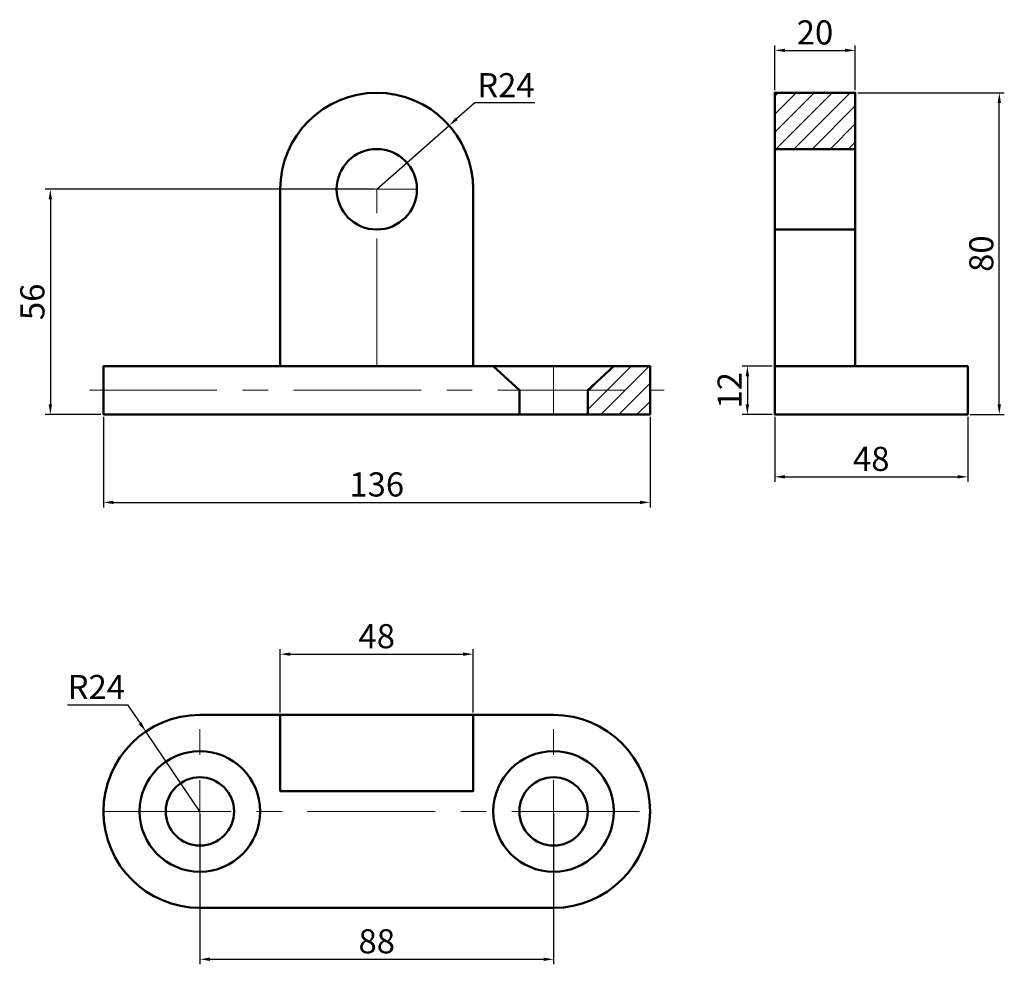
# Model space of a CAD drawing. Units: millimetres. Extents: x 11 to 256, y 19 to 254.
import ezdxf

# ---------------------------------------------------------------- set-up
doc = ezdxf.new("R2010")
doc.units = ezdxf.units.MM
doc.linetypes.add('CENTER', pattern=[50.8, 31.75, -6.35, 6.35, -6.35])
for name, color, linetype, lineweight in [('M-CNTR', 1, 'CENTER', 18), ('M-DIMS', 2, 'Continuous', 25), ('M-HATC', 8, 'Continuous', 18), ('M-OUTL', 7, 'Continuous', 50)]:
    doc.layers.add(name, color=color, linetype=linetype, lineweight=lineweight)
doc.styles.get("Standard").update_dxf_attribs({"font": 'arial.ttf'})
doc.dimstyles.new('ISO-25', dxfattribs={"dimtxt": 6, "dimasz": 2.5, "dimexe": 1.25, "dimexo": 0.625, "dimtad": 1, "dimtoh": 1, "dimdec": 0, "dimtxsty": 'Standard', "dimcen": 2.5, "dimadec": 0, "dimazin": 0, "dimtfac": 1, "dimtdec": 0, "dimtmove": 0, "dimatfit": 3, "dimfxl": 1, "dimarcsym": 0})

# ---------------------------------------------------------------- blocks, each defined once
blk = doc.blocks.new('*D1')
at = {"layer": 'Defpoints', "color": 0, "transparency": 16777216}
for p in [(32.29, 156.06), (168.29, 156.06), (168.29, 134.17)]:
    blk.add_point(p, dxfattribs=at)
at = {"layer": 'M-DIMS', "color": 0, "lineweight": -2, "transparency": 16777216}
for p, q in [((32.29, 155.44), (32.29, 132.92)), ((168.29, 155.44), (168.29, 132.92)), ((34.79, 134.17), (165.79, 134.17))]:
    blk.add_line(p, q, dxfattribs=at)
at = {"layer": 'M-DIMS', "color": 0, "transparency": 16777216}
for points in [[(34.79, 134.59), (34.79, 133.76), (32.29, 134.17)], [(165.79, 134.59), (165.79, 133.76), (168.29, 134.17)]]:
    blk.add_solid(points, dxfattribs=at)
at = {"layer": 'M-DIMS', "color": 0, "transparency": 16777216, "insert": (100.29, 137.86), "char_height": 6, "attachment_point": 5}
blk.add_mtext('136', dxfattribs=at)
blk = doc.blocks.new('*D2')
at = {"layer": 'Defpoints', "color": 0, "transparency": 16777216}
for p in [(118.29, 227.93), (100.29, 212.06)]:
    blk.add_point(p, dxfattribs=at)
at = {"layer": 'M-DIMS', "color": 0, "lineweight": -2, "transparency": 16777216}
for p, q in [((124.66, 233.54), (120.17, 229.58)), ((139.6, 233.54), (124.66, 233.54)), ((100.29, 212.06), (118.29, 227.93))]:
    blk.add_line(p, q, dxfattribs=at)
at = {"layer": 'M-DIMS', "color": 0, "transparency": 16777216}
blk.add_solid([(119.89, 229.9), (120.44, 229.27), (118.29, 227.93)], dxfattribs=at)
at = {"layer": 'M-DIMS', "color": 0, "transparency": 16777216, "insert": (132.44, 237.18), "char_height": 6, "attachment_point": 5}
blk.add_mtext('R24', dxfattribs=at)
blk = doc.blocks.new('*D3')
at = {"layer": 'Defpoints', "color": 0, "transparency": 16777216}
for p in [(199.33, 156.06), (247.33, 156.06), (247.33, 140.53)]:
    blk.add_point(p, dxfattribs=at)
at = {"layer": 'M-DIMS', "color": 0, "lineweight": -2, "transparency": 16777216}
for p, q in [((199.33, 155.44), (199.33, 139.28)), ((247.33, 155.44), (247.33, 139.28)), ((201.83, 140.53), (244.83, 140.53))]:
    blk.add_line(p, q, dxfattribs=at)
at = {"layer": 'M-DIMS', "color": 0, "transparency": 16777216}
for points in [[(201.83, 140.95), (201.83, 140.12), (199.33, 140.53)], [(244.83, 140.95), (244.83, 140.12), (247.33, 140.53)]]:
    blk.add_solid(points, dxfattribs=at)
at = {"layer": 'M-DIMS', "color": 0, "transparency": 16777216, "insert": (223.33, 144.22), "char_height": 6, "attachment_point": 5}
blk.add_mtext('48', dxfattribs=at)
blk = doc.blocks.new('*D4')
at = {"layer": 'Defpoints', "color": 0, "transparency": 16777216}
for p in [(219.33, 246.62), (199.33, 236.06), (219.33, 236.06)]:
    blk.add_point(p, dxfattribs=at)
at = {"layer": 'M-DIMS', "color": 0, "lineweight": -2, "transparency": 16777216}
for p, q in [((199.33, 236.69), (199.33, 247.87)), ((219.33, 236.69), (219.33, 247.87)), ((201.83, 246.62), (216.83, 246.62))]:
    blk.add_line(p, q, dxfattribs=at)
at = {"layer": 'M-DIMS', "color": 0, "transparency": 16777216}
for points in [[(201.83, 247.04), (201.83, 246.21), (199.33, 246.62)], [(216.83, 247.04), (216.83, 246.21), (219.33, 246.62)]]:
    blk.add_solid(points, dxfattribs=at)
at = {"layer": 'M-DIMS', "color": 0, "transparency": 16777216, "insert": (209.33, 250.31), "char_height": 6, "attachment_point": 5}
blk.add_mtext('20', dxfattribs=at)
blk = doc.blocks.new('*D5')
at = {"layer": 'Defpoints', "color": 0, "transparency": 16777216}
for p in [(219.33, 236.06), (255.18, 236.06), (247.33, 156.06)]:
    blk.add_point(p, dxfattribs=at)
at = {"layer": 'M-DIMS', "color": 0, "lineweight": -2, "transparency": 16777216}
for p, q in [((219.96, 236.06), (256.43, 236.06)), ((255.18, 158.56), (255.18, 233.56)), ((247.96, 156.06), (256.43, 156.06))]:
    blk.add_line(p, q, dxfattribs=at)
at = {"layer": 'M-DIMS', "color": 0, "transparency": 16777216}
for points in [[(254.77, 233.56), (255.6, 233.56), (255.18, 236.06)], [(254.77, 158.56), (255.6, 158.56), (255.18, 156.06)]]:
    blk.add_solid(points, dxfattribs=at)
at = {"layer": 'M-DIMS', "color": 0, "transparency": 16777216, "insert": (251.49, 196.06), "char_height": 6, "attachment_point": 5, "rotation": 90}
blk.add_mtext('80', dxfattribs=at)
blk = doc.blocks.new('*D6')
at = {"layer": 'Defpoints', "color": 0, "transparency": 16777216}
for p in [(199.33, 168.06), (192.5, 156.06), (199.33, 156.06)]:
    blk.add_point(p, dxfattribs=at)
at = {"layer": 'M-DIMS', "color": 0, "lineweight": -2, "transparency": 16777216}
for p, q in [((198.71, 168.06), (191.25, 168.06)), ((192.5, 165.56), (192.5, 158.56)), ((198.71, 156.06), (191.25, 156.06))]:
    blk.add_line(p, q, dxfattribs=at)
at = {"layer": 'M-DIMS', "color": 0, "transparency": 16777216}
for points in [[(192.08, 165.56), (192.92, 165.56), (192.5, 168.06)], [(192.08, 158.56), (192.92, 158.56), (192.5, 156.06)]]:
    blk.add_solid(points, dxfattribs=at)
at = {"layer": 'M-DIMS', "color": 0, "transparency": 16777216, "insert": (188.86, 162.06), "char_height": 6, "attachment_point": 5, "rotation": 90}
blk.add_mtext('12', dxfattribs=at)
blk = doc.blocks.new('*D7')
at = {"layer": 'Defpoints', "color": 0, "transparency": 16777216}
for p in [(124.29, 96.42), (76.29, 81.3), (124.29, 81.3)]:
    blk.add_point(p, dxfattribs=at)
at = {"layer": 'M-DIMS', "color": 0, "lineweight": -2, "transparency": 16777216}
for p, q in [((76.29, 81.93), (76.29, 97.67)), ((78.79, 96.42), (121.79, 96.42)), ((124.29, 81.93), (124.29, 97.67))]:
    blk.add_line(p, q, dxfattribs=at)
at = {"layer": 'M-DIMS', "color": 0, "transparency": 16777216}
for points in [[(78.79, 96.84), (78.79, 96.01), (76.29, 96.42)], [(121.79, 96.84), (121.79, 96.01), (124.29, 96.42)]]:
    blk.add_solid(points, dxfattribs=at)
at = {"layer": 'M-DIMS', "color": 0, "transparency": 16777216, "insert": (100.29, 100.11), "char_height": 6, "attachment_point": 5}
blk.add_mtext('48', dxfattribs=at)
blk = doc.blocks.new('*D8')
at = {"layer": 'Defpoints', "color": 0, "transparency": 16777216}
for p in [(100.29, 212.06), (19.08, 156.06), (32.29, 156.06)]:
    blk.add_point(p, dxfattribs=at)
at = {"layer": 'M-DIMS', "color": 0, "lineweight": -2, "transparency": 16777216}
for p, q in [((99.66, 212.06), (17.83, 212.06)), ((19.08, 209.56), (19.08, 158.56)), ((31.66, 156.06), (17.83, 156.06))]:
    blk.add_line(p, q, dxfattribs=at)
at = {"layer": 'M-DIMS', "color": 0, "transparency": 16777216}
for points in [[(18.66, 209.56), (19.5, 209.56), (19.08, 212.06)], [(18.66, 158.56), (19.5, 158.56), (19.08, 156.06)]]:
    blk.add_solid(points, dxfattribs=at)
at = {"layer": 'M-DIMS', "color": 0, "transparency": 16777216, "insert": (15.39, 184.06), "char_height": 6, "attachment_point": 5, "rotation": 90}
blk.add_mtext('56', dxfattribs=at)
blk = doc.blocks.new('*D9')
at = {"layer": 'Defpoints', "color": 0, "transparency": 16777216}
for p in [(42.83, 77.17), (56.29, 57.3)]:
    blk.add_point(p, dxfattribs=at)
at = {"layer": 'M-DIMS', "color": 0, "lineweight": -2, "transparency": 16777216}
for p, q in [((23.37, 83.85), (38.31, 83.85)), ((38.31, 83.85), (41.43, 79.24)), ((56.29, 57.3), (42.83, 77.17))]:
    blk.add_line(p, q, dxfattribs=at)
at = {"layer": 'M-DIMS', "color": 0, "transparency": 16777216}
blk.add_solid([(41.77, 79.48), (41.08, 79.01), (42.83, 77.17)], dxfattribs=at)
at = {"layer": 'M-DIMS', "color": 0, "transparency": 16777216, "insert": (30.53, 87.48), "char_height": 6, "attachment_point": 5}
blk.add_mtext('R24', dxfattribs=at)
blk = doc.blocks.new('*D10')
at = {"layer": 'Defpoints', "color": 0, "transparency": 16777216}
for p in [(56.29, 57.3), (144.29, 57.3), (144.29, 20.52)]:
    blk.add_point(p, dxfattribs=at)
at = {"layer": 'M-DIMS', "color": 0, "lineweight": -2, "transparency": 16777216}
for p, q in [((56.29, 56.68), (56.29, 19.27)), ((144.29, 56.68), (144.29, 19.27)), ((58.79, 20.52), (141.79, 20.52))]:
    blk.add_line(p, q, dxfattribs=at)
at = {"layer": 'M-DIMS', "color": 0, "transparency": 16777216}
for points in [[(58.79, 20.94), (58.79, 20.1), (56.29, 20.52)], [(141.79, 20.94), (141.79, 20.1), (144.29, 20.52)]]:
    blk.add_solid(points, dxfattribs=at)
at = {"layer": 'M-DIMS', "color": 0, "transparency": 16777216, "insert": (100.29, 24.21), "char_height": 6, "attachment_point": 5}
blk.add_mtext('88', dxfattribs=at)
blk = doc.blocks.new('HOLE-CSK-17')
for radius in [15, 8.5]:
    blk.add_circle((56.29, 57.3), radius)

msp = doc.modelspace()

# ---------------------------------------------------------------- hatches: boundary and pattern name
at = {"layer": 'M-HATC'}
h = msp.add_hatch(dxfattribs=at)
h.set_pattern_fill('ANSI31', color=256)
h.paths.add_polyline_path([(219.33, 236.06), (199.33, 236.06), (199.33, 222.06), (219.33, 222.06)])
h.paths.add_polyline_path([(168.29, 168.06), (159.29, 168.06), (152.79, 162.06), (168.29, 162.06)])
h.paths.add_polyline_path([(168.29, 162.06), (152.79, 162.06), (152.79, 156.06), (168.29, 156.06)])

# ---------------------------------------------------------------- linework, layer by layer
at = {"layer": 'M-CNTR'}
for p, q in [((90.29, 212.06), (110.29, 212.06)), ((100.29, 168.06), (100.29, 212.06)), ((144.29, 156.06), (144.29, 168.06)), ((28.79, 162.06), (171.79, 162.06)), ((56.29, 33.3), (56.29, 81.3)), ((144.29, 33.3), (144.29, 81.3)), ((32.29, 57.3), (168.29, 57.3))]:
    msp.add_line(p, q, dxfattribs=at)
at = {"layer": 'M-OUTL'}
for p, q in [((199.33, 222.06), (219.33, 222.06)), ((199.33, 202.06), (219.33, 202.06))]:
    msp.add_line(p, q, dxfattribs=at)
msp.add_lwpolyline([(76.29, 168.06), (76.29, 212.06, -1), (124.29, 212.06), (124.29, 168.06)], format="xyb", dxfattribs=at)
for points in [[(199.33, 168.06), (247.33, 168.06), (247.33, 156.06), (199.33, 156.06), (199.33, 168.06), (199.33, 236.06), (219.33, 236.06), (219.33, 168.06)], [(129.29, 168.06), (135.79, 162.06), (135.79, 156.06)], [(152.79, 156.06), (152.79, 162.06), (159.29, 168.06)], [(76.29, 81.3), (76.29, 62.35), (124.29, 62.35), (124.29, 81.3)]]:
    msp.add_lwpolyline(points, dxfattribs=at)
msp.add_lwpolyline([(32.29, 156.06), (32.29, 168.06), (168.29, 168.06), (168.29, 156.06)], close=True, dxfattribs=at)
msp.add_lwpolyline([(56.29, 33.3), (144.29, 33.3, 1), (144.29, 81.3), (56.29, 81.3, 1)], format="xyb", close=True, dxfattribs=at)
msp.add_circle((100.29, 212.06), 10, dxfattribs=at)

# ---------------------------------------------------------------- block references
for p in [(0, 0), (88, 0)]:
    msp.add_blockref('HOLE-CSK-17', p, dxfattribs=at)

# ---------------------------------------------------------------- dimensions: what is measured, and where the dimension line sits
at = {"layer": 'M-DIMS'}
for base, p1, p2, picture, middle in [((219.33, 246.62), (199.33, 236.06), (219.33, 236.06), '*D4', (209.33, 250.31)), ((168.29, 134.17), (32.29, 156.06), (168.29, 156.06), '*D1', (100.29, 137.86)), ((247.33, 140.53), (199.33, 156.06), (247.33, 156.06), '*D3', (223.33, 144.22)), ((124.29, 96.42), (76.29, 81.3), (124.29, 81.3), '*D7', (100.29, 100.11)), ((144.29, 20.52), (56.29, 57.3), (144.29, 57.3), '*D10', (100.29, 24.21))]:
    dim = msp.add_linear_dim(base=base, p1=p1, p2=p2, dimstyle='ISO-25', override={"dimclrd": 0, "dimclre": 0, "dimclrt": 0}, dxfattribs=at)
    dim.commit()
    dim.dimension.update_dxf_attribs({"geometry": picture, "text_midpoint": middle})
for center, mpoint, picture, middle in [((100.29, 212.06), (118.29, 227.93), '*D2', (132.44, 233.54)), ((56.29, 57.3), (42.83, 77.17), '*D9', (30.53, 83.85))]:
    dim = msp.add_radius_dim(center=center, mpoint=mpoint, dimstyle='ISO-25', override={"dimclrd": 0, "dimclre": 0, "dimclrt": 0}, dxfattribs=at)
    dim.commit()
    dim.dimension.update_dxf_attribs({"geometry": picture, "text_midpoint": middle, "dimtype": 164})
for base, p1, p2, picture, middle in [((255.18, 236.06), (247.33, 156.06), (219.33, 236.06), '*D5', (251.49, 196.06)), ((19.08, 156.06), (100.29, 212.06), (32.29, 156.06), '*D8', (15.39, 184.06)), ((192.5, 156.06), (199.33, 168.06), (199.33, 156.06), '*D6', (188.86, 162.06))]:
    dim = msp.add_linear_dim(base=base, p1=p1, p2=p2, angle=90, dimstyle='ISO-25', override={"dimclrd": 0, "dimclre": 0, "dimclrt": 0}, dxfattribs=at)
    dim.commit()
    dim.dimension.update_dxf_attribs({"geometry": picture, "text_midpoint": middle})

doc.saveas('drawing.dxf')
